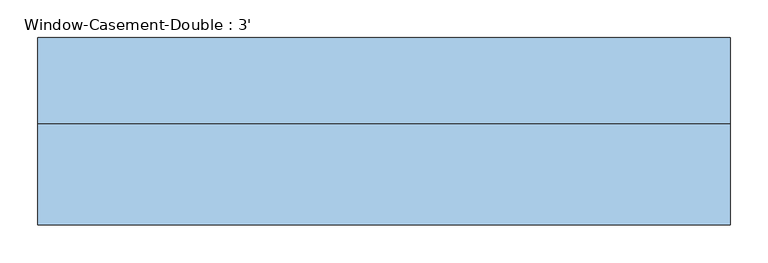
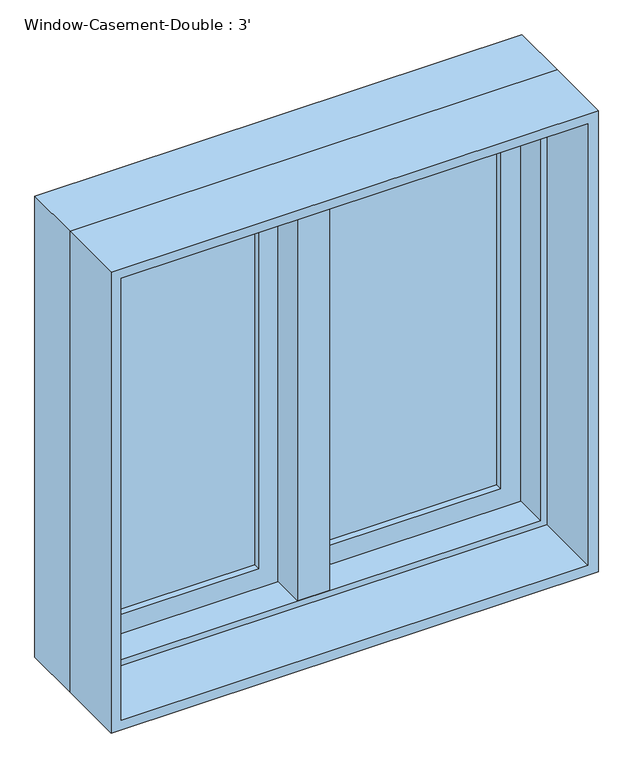
"""IFC4 building model written with IfcOpenShell, lengths in millimetres: window geometry, Window-Casement-Double : 3'."""

from ifc_helpers import new_model, si_unit, frame, origin, place, context, project, spatial, polyline, outline, extrude, faceted_brep, source, transform, mapped, element, save


def window_casement_double_3_90de19e9(model_context):
    return source(origin(), model_context, "Body", "SolidModel", [
        faceted_brep([(9.525, 133.35, 1816.1), (-9.525, 133.35, 1816.1), (-9.525, 82.55, 1816.1), (9.525, 82.55, 1816.1), (9.525, 133.35, 927.1), (9.525, 82.55, 927.1), (-9.525, 82.55, 927.1), (-9.525, 133.35, 927.1), (-9.525, 82.55, 946.15), (-9.525, 82.55, 1797.05), (-30.1625, 82.55, 946.15), (-30.1625, 82.55, 1797.05), (-30.1625, 19.05, 946.15), (-30.1625, 19.05, 1797.05), (30.1625, 19.05, 946.15), (30.1625, 19.05, 1797.05), (30.1625, 82.55, 946.15), (30.1625, 82.55, 1797.05), (9.525, 82.55, 946.15), (9.525, 82.55, 1797.05)], [[[0, 1, 2, 3]], [[4, 5, 6, 7]], [[1, 0, 4, 7]], [[2, 1, 7, 6, 8, 9]], [[9, 8, 10, 11]], [[11, 10, 12, 13]], [[13, 12, 14, 15]], [[15, 14, 16, 17]], [[17, 16, 18, 19]], [[0, 3, 19, 18, 5, 4]], [[18, 8, 6, 5]], [[9, 19, 3, 2]], [[8, 18, 16, 14, 12, 10]], [[19, 9, 11, 13, 15, 17]]]),
        extrude(outline(polyline([(-66.675, 114.3), (-66.675, 107.95), (-387.35, 107.95), (-387.35, 114.3), (-66.675, 114.3)])), frame((0.0, 0.0, 984.25), z_axis=(0.0, 0.0, 1.0), x_axis=(1.0, 0.0, 0.0)), (0.0, 0.0, 1.0), 774.7),
        extrude(outline(polyline([(-387.35, 95.25), (-387.35, 101.6), (-66.675, 101.6), (-66.675, 95.25), (-387.35, 95.25)])), frame((0.0, 0.0, 984.25), z_axis=(0.0, 0.0, 1.0), x_axis=(1.0, 0.0, 0.0)), (0.0, 0.0, 1.0), 774.7),
        extrude(outline(polyline([(387.35, 114.3), (387.35, 107.95), (66.675, 107.95), (66.675, 114.3), (387.35, 114.3)])), frame((0.0, 0.0, 984.25), z_axis=(0.0, 0.0, 1.0), x_axis=(1.0, 0.0, 0.0)), (0.0, 0.0, 1.0), 774.7),
        extrude(outline(polyline([(66.675, 95.25), (66.675, 101.6), (387.35, 101.6), (387.35, 95.25), (66.675, 95.25)])), frame((0.0, 0.0, 984.25), z_axis=(0.0, 0.0, 1.0), x_axis=(1.0, 0.0, 0.0)), (0.0, 0.0, 1.0), 774.7),
        extrude(outline(polyline([(1816.1, -444.5), (927.1, -444.5), (927.1, -9.525), (1816.1, -9.525), (1816.1, -444.5)]), holes=[polyline([(1758.95, -66.675), (984.25, -66.675), (984.25, -387.35), (1758.95, -387.35), (1758.95, -66.675)])]), frame((0.0, 82.55, 0.0), z_axis=(0.0, 1.0, 0.0), x_axis=(0.0, 0.0, 1.0)), (0.0, 0.0, 1.0), 44.45),
        extrude(outline(polyline([(927.1, 444.5), (1816.1, 444.5), (1816.1, 9.525), (927.1, 9.525), (927.1, 444.5)]), holes=[polyline([(984.25, 66.675), (1758.95, 66.675), (1758.95, 387.35), (984.25, 387.35), (984.25, 66.675)])]), frame((0.0, 82.55, 0.0), z_axis=(0.0, 1.0, 0.0), x_axis=(0.0, 0.0, 1.0)), (0.0, 0.0, 1.0), 44.45),
        extrude(outline(polyline([(1828.8, -457.2), (914.4, -457.2), (914.4, 457.2), (1828.8, 457.2), (1828.8, -457.2)]), holes=[polyline([(1809.75, 438.15), (933.45, 438.15), (933.45, -438.15), (1809.75, -438.15), (1809.75, 438.15)])]), frame((0.0, -114.3, 0.0), z_axis=(0.0, 1.0, 0.0), x_axis=(0.0, 0.0, 1.0)), (0.0, 0.0, 1.0), 133.35),
        faceted_brep([(425.45, 82.55, 1797.05), (425.45, 19.05, 1797.05), (-425.45, 19.05, 1797.05), (-425.45, 82.55, 1797.05), (444.5, 133.35, 1816.1), (444.5, 82.55, 1816.1), (-444.5, 82.55, 1816.1), (-444.5, 133.35, 1816.1), (457.2, 19.05, 1828.8), (457.2, 133.35, 1828.8), (-457.2, 133.35, 1828.8), (-457.2, 19.05, 1828.8), (-425.45, 19.05, 946.15), (-425.45, 82.55, 946.15), (-444.5, 82.55, 927.1), (-444.5, 133.35, 927.1), (-457.2, 133.35, 914.4), (-457.2, 19.05, 914.4), (425.45, 19.05, 946.15), (425.45, 82.55, 946.15), (444.5, 82.55, 927.1), (444.5, 133.35, 927.1), (457.2, 133.35, 914.4), (457.2, 19.05, 914.4)], [[[0, 1, 2, 3]], [[4, 5, 6, 7]], [[8, 9, 10, 11]], [[3, 2, 12, 13]], [[7, 6, 14, 15]], [[11, 10, 16, 17]], [[13, 12, 18, 19]], [[15, 14, 20, 21]], [[17, 16, 22, 23]], [[11, 17, 23, 8], [1, 18, 12, 2]], [[19, 18, 1, 0]], [[5, 20, 14, 6], [3, 13, 19, 0]], [[21, 20, 5, 4]], [[23, 22, 9, 8]], [[9, 22, 16, 10], [7, 15, 21, 4]]]),
    ])


if __name__ == "__main__":
    model = new_model("IFC4")
    model_context = context("Model", 3, world=origin())
    ifc_project = project(units=[si_unit("LENGTHUNIT", "METRE", prefix="MILLI")], contexts=[model_context])
    site = spatial("IfcSite", under=ifc_project)
    building = spatial("IfcBuilding", under=site)
    placement = place(None, origin())
    window_casement_double_3_shape = window_casement_double_3_90de19e9(model_context)
    element("IfcWindow", 1, ObjectType="Window-Casement-Double : 3'", at=placement, inside=building, context=model_context, shape_type="MappedRepresentation", body=[
        mapped(window_casement_double_3_shape, transform((0.0, 0.0, 0.0), x_axis=(1.0, 0.0, 0.0), y_axis=(0.0, 1.0, 0.0), z_axis=(0.0, 0.0, 1.0))),
    ])
    save(model, "model.ifc")

# Revit data of these elements
# Type "Window-Casement-Double : 3'"
#   Type Mark = "19"
#   Fire Rating = "0.5h"
#   Assembly Code = "B2020100"
#   Analytic Construction = "Double glazing - domestic"
#   Frame Extension [instance default] = 0' - 0 1/4"
#   Window Inset [instance default] = 0' - 0"
#   Wall Thickness [instance default] = 0' - 6"
#   Interior Wall Closure [instance default] = 0' - 2 1/4"
#   Half Width = 1' - 6"
#   Visual Light Transmittance = 0.81
#   Thermal Resistance (R) = 1.8146 (h·ft²·°F)/BTU
#   Solar Heat Gain Coefficient = 0.76
#   Rough Width = 3' - 0 1/2"
#   Rough Height = 3' - 0 1/2"
#   Height = 3' - 0"
#   Heat Transfer Coefficient (U) = 0.5511 BTU/(h·ft²·°F)
#   Exterior Wall Closure [instance default] = 0' - 1 1/4"
#   Extension Jamb [instance default] = 0' - 2 1/4"
#   Default Sill Height = 3' - 0"
#   Width = 3' - 0"
#   Muntin Visibility = yes
#   Interior Trim Visibility [instance default] = yes
#   Exterior Trim Visibility [instance default] = yes
#   Extension Jamb Visibility [instance default] = yes
#   Interior Trim Material = Wood - Stained
#   Muntin Pattern = Muntin Pattern_2x2 : Muntin Pattern_2x2
#   Interior Trim = Trim-Window-Interior-Flat : Picture Frame
#   Interior Frame Material = Wood - Stained
#   Glass Panel Material = Glass
#   Exterior Trim Material = Clad - White
#   Exterior Trim = Trim-Window-Exterior-Flat : with Sill
#   Exterior Frame Material = Clad - White
#   Wall Closure = (empty or 0)
# Element 1 (IfcWindow, "Window-Casement-Double : 3'")
#   Wall Thickness = 0' - 9"
#   Extension Jamb = 0' - 5 1/4"
#   Materials on its faces: "Wood - Stained", "Glass", "Clad - White"
# Materials
#   "Wood - Stained": class "Wood", colour RGB 224 178 126, transparency 0, Cost = 0
#   "Glass": class "Glass", colour RGB 0 128 192, transparency 0.75, Description = "Soda Lime Glass", Cost = 0
#   "Clad - White": class "Wood", colour RGB 242 242 238, transparency 0, Cost = 0
